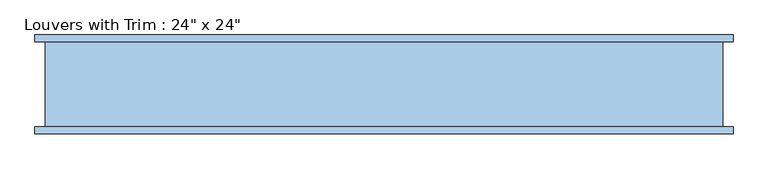
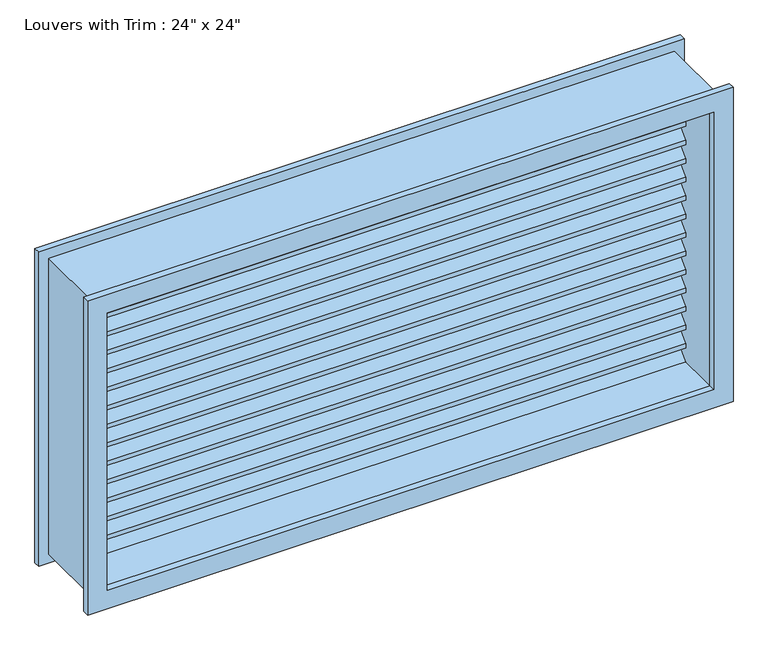
"""IFC4 building model written with IfcOpenShell, lengths in millimetres: window geometry."""

from ifc_helpers import new_model, si_unit, frame, origin, place, context, project, spatial, polyline, outline, extrude, source, transform, mapped, element, save


def window_67e7833d(model_context):
    return source(origin(), model_context, "Body", "SweptSolid", [
        extrude(outline(polyline([(1543.05, -628.65), (895.35, -628.65), (895.35, 628.65), (1543.05, 628.65), (1543.05, -628.65)]), holes=[polyline([(1504.95, -590.55), (1504.95, 590.55), (933.45, 590.55), (933.45, -590.55), (1504.95, -590.55)])]), frame((0.0, 69.85, 0.0), z_axis=(0.0, 1.0, 0.0), x_axis=(0.0, 0.0, 1.0)), (0.0, 0.0, 1.0), 12.7),
        extrude(outline(polyline([(1543.05, 628.65), (1543.05, -628.65), (895.35, -628.65), (895.35, 628.65), (1543.05, 628.65)]), holes=[polyline([(1504.95, 590.55), (933.45, 590.55), (933.45, -590.55), (1504.95, -590.55), (1504.95, 590.55)])]), frame((0.0, -95.25, 0.0), z_axis=(0.0, 1.0, 0.0), x_axis=(0.0, 0.0, 1.0)), (0.0, 0.0, 1.0), 12.7),
        extrude(outline(polyline([(1524.0, 609.6), (1524.0, -609.6), (914.4, -609.6), (914.4, 609.6), (1524.0, 609.6)]), holes=[polyline([(1504.95, 590.55), (933.45, 590.55), (933.45, -590.55), (1504.95, -590.55), (1504.95, 590.55)])]), frame((0.0, -82.55, 0.0), z_axis=(0.0, 1.0, 0.0), x_axis=(0.0, 0.0, 1.0)), (0.0, 0.0, 1.0), 152.4),
        extrude(outline(polyline([(33.9289755, 969.3710245), (69.85, 933.45), (60.8697439, 933.45), (33.9289755, 960.3907684), (6.9882072, 933.45), (-1.992049, 933.45), (33.9289755, 969.3710245)])), frame((-590.55, 0.0, 0.0), z_axis=(1.0, 0.0, 0.0), x_axis=(0.0, 1.0, 0.0)), (0.0, 0.0, 1.0), 1181.1),
        extrude(outline(polyline([(33.9289755, 1007.4710245), (69.85, 971.55), (69.85, 962.5697439), (33.9289755, 998.4907684), (-1.992049, 962.5697439), (-1.992049, 971.55), (33.9289755, 1007.4710245)])), frame((-590.55, 0.0, 0.0), z_axis=(1.0, 0.0, 0.0), x_axis=(0.0, 1.0, 0.0)), (0.0, 0.0, 1.0), 1181.1),
        extrude(outline(polyline([(33.9289755, 1045.5710245), (69.85, 1009.65), (69.85, 1000.6697439), (33.9289755, 1036.5907684), (-1.992049, 1000.6697439), (-1.992049, 1009.65), (33.9289755, 1045.5710245)])), frame((-590.55, 0.0, 0.0), z_axis=(1.0, 0.0, 0.0), x_axis=(0.0, 1.0, 0.0)), (0.0, 0.0, 1.0), 1181.1),
        extrude(outline(polyline([(33.9289755, 1083.6710245), (69.85, 1047.75), (69.85, 1038.7697439), (33.9289755, 1074.6907684), (-1.992049, 1038.7697439), (-1.992049, 1047.75), (33.9289755, 1083.6710245)])), frame((-590.55, 0.0, 0.0), z_axis=(1.0, 0.0, 0.0), x_axis=(0.0, 1.0, 0.0)), (0.0, 0.0, 1.0), 1181.1),
        extrude(outline(polyline([(33.9289755, 1121.7710245), (69.85, 1085.85), (69.85, 1076.8697439), (33.9289755, 1112.7907684), (-1.992049, 1076.8697439), (-1.992049, 1085.85), (33.9289755, 1121.7710245)])), frame((-590.55, 0.0, 0.0), z_axis=(1.0, 0.0, 0.0), x_axis=(0.0, 1.0, 0.0)), (0.0, 0.0, 1.0), 1181.1),
        extrude(outline(polyline([(33.9289755, 1159.8710245), (69.85, 1123.95), (69.85, 1114.9697439), (33.9289755, 1150.8907684), (-1.992049, 1114.9697439), (-1.992049, 1123.95), (33.9289755, 1159.8710245)])), frame((-590.55, 0.0, 0.0), z_axis=(1.0, 0.0, 0.0), x_axis=(0.0, 1.0, 0.0)), (0.0, 0.0, 1.0), 1181.1),
        extrude(outline(polyline([(33.9289755, 1197.9710245), (69.85, 1162.05), (69.85, 1153.0697439), (33.9289755, 1188.9907684), (-1.992049, 1153.0697439), (-1.992049, 1162.05), (33.9289755, 1197.9710245)])), frame((-590.55, 0.0, 0.0), z_axis=(1.0, 0.0, 0.0), x_axis=(0.0, 1.0, 0.0)), (0.0, 0.0, 1.0), 1181.1),
        extrude(outline(polyline([(33.9289755, 1236.0710245), (69.85, 1200.15), (69.85, 1191.1697439), (33.9289755, 1227.0907684), (-1.992049, 1191.1697439), (-1.992049, 1200.15), (33.9289755, 1236.0710245)])), frame((-590.55, 0.0, 0.0), z_axis=(1.0, 0.0, 0.0), x_axis=(0.0, 1.0, 0.0)), (0.0, 0.0, 1.0), 1181.1),
        extrude(outline(polyline([(33.9289755, 1274.1710245), (69.85, 1238.25), (69.85, 1229.2697439), (33.9289755, 1265.1907684), (-1.992049, 1229.2697439), (-1.992049, 1238.25), (33.9289755, 1274.1710245)])), frame((-590.55, 0.0, 0.0), z_axis=(1.0, 0.0, 0.0), x_axis=(0.0, 1.0, 0.0)), (0.0, 0.0, 1.0), 1181.1),
        extrude(outline(polyline([(33.9289755, 1312.2710245), (69.85, 1276.35), (69.85, 1267.3697439), (33.9289755, 1303.2907684), (-1.992049, 1267.3697439), (-1.992049, 1276.35), (33.9289755, 1312.2710245)])), frame((-590.55, 0.0, 0.0), z_axis=(1.0, 0.0, 0.0), x_axis=(0.0, 1.0, 0.0)), (0.0, 0.0, 1.0), 1181.1),
        extrude(outline(polyline([(33.9289755, 1350.3710245), (69.85, 1314.45), (69.85, 1305.4697439), (33.9289755, 1341.3907684), (-1.992049, 1305.4697439), (-1.992049, 1314.45), (33.9289755, 1350.3710245)])), frame((-590.55, 0.0, 0.0), z_axis=(1.0, 0.0, 0.0), x_axis=(0.0, 1.0, 0.0)), (0.0, 0.0, 1.0), 1181.1),
        extrude(outline(polyline([(33.9289755, 1388.4710245), (69.85, 1352.55), (69.85, 1343.5697439), (33.9289755, 1379.4907684), (-1.992049, 1343.5697439), (-1.992049, 1352.55), (33.9289755, 1388.4710245)])), frame((-590.55, 0.0, 0.0), z_axis=(1.0, 0.0, 0.0), x_axis=(0.0, 1.0, 0.0)), (0.0, 0.0, 1.0), 1181.1),
        extrude(outline(polyline([(33.9289755, 1426.5710245), (69.85, 1390.65), (69.85, 1381.6697439), (33.9289755, 1417.5907684), (-1.992049, 1381.6697439), (-1.992049, 1390.65), (33.9289755, 1426.5710245)])), frame((-590.55, 0.0, 0.0), z_axis=(1.0, 0.0, 0.0), x_axis=(0.0, 1.0, 0.0)), (0.0, 0.0, 1.0), 1181.1),
        extrude(outline(polyline([(33.9289755, 1464.6710245), (69.85, 1428.75), (69.85, 1419.7697439), (33.9289755, 1455.6907684), (-1.992049, 1419.7697439), (-1.992049, 1428.75), (33.9289755, 1464.6710245)])), frame((-590.55, 0.0, 0.0), z_axis=(1.0, 0.0, 0.0), x_axis=(0.0, 1.0, 0.0)), (0.0, 0.0, 1.0), 1181.1),
        extrude(outline(polyline([(33.9289755, 1502.7710245), (69.85, 1466.85), (69.85, 1457.8697439), (33.9289755, 1493.7907684), (-1.992049, 1457.8697439), (-1.992049, 1466.85), (33.9289755, 1502.7710245)])), frame((-590.55, 0.0, 0.0), z_axis=(1.0, 0.0, 0.0), x_axis=(0.0, 1.0, 0.0)), (0.0, 0.0, 1.0), 1181.1),
    ])


if __name__ == "__main__":
    model = new_model("IFC4")
    model_context = context("Model", 3, world=origin())
    ifc_project = project(units=[si_unit("LENGTHUNIT", "METRE", prefix="MILLI")], contexts=[model_context])
    site = spatial("IfcSite", under=ifc_project)
    building = spatial("IfcBuilding", under=site)
    placement = place(None, origin())
    window_shape = window_67e7833d(model_context)
    element("IfcWindow", 1, ObjectType="Louvers with Trim : 24\" x 24\"", at=placement, inside=building, context=model_context, shape_type="MappedRepresentation", body=[
        mapped(window_shape, transform((0.0, 0.0, 0.0), x_axis=(1.0, 0.0, 0.0), y_axis=(0.0, 1.0, 0.0), z_axis=(0.0, 0.0, 1.0))),
    ])
    save(model, "model.ifc")

# Revit data of these elements
# Type "Louvers with Trim : 24\" x 24\""
#   Type Mark = "26"
#   Construction Type Id = "GSP4R"
#   Assembly Code = "B20"
#   Analytic Construction = "1/8 in Pilkington single glazing"
#   Visual Light Transmittance = 0.9
#   Solar Heat Gain Coefficient = 0.78
#   Heat Transfer Coefficient (U) = 0.6496 BTU/(h·ft²·°F)
#   Default Sill Height = 3' - 0"
#   Trim Projection - Ext. = 0' - 0 1/2"
#   Trim Projection - Int. = 0' - 0 1/2"
#   Trim Width - Exterior = 0' - 1 1/2"
#   Trim Width - Interior = 0' - 1 1/2"
#   Width = 4' - 0"
#   Define Thermal Properties by = 1
#   Frame Material = Birch
#   Louver Material = Birch
#   Trim Exterior Material = Birch
#   Trim Interior Material = Birch
#   Wall Closure = (empty or 0)
# Element 1 (IfcWindow, "Louvers with Trim : 24\" x 24\"")
#   Materials on its faces: "Birch"
# Materials
#   "Birch": class "Wood", colour RGB 224 178 126, transparency 0, Description = "Betula Alleghaniensis", Cost = 0
